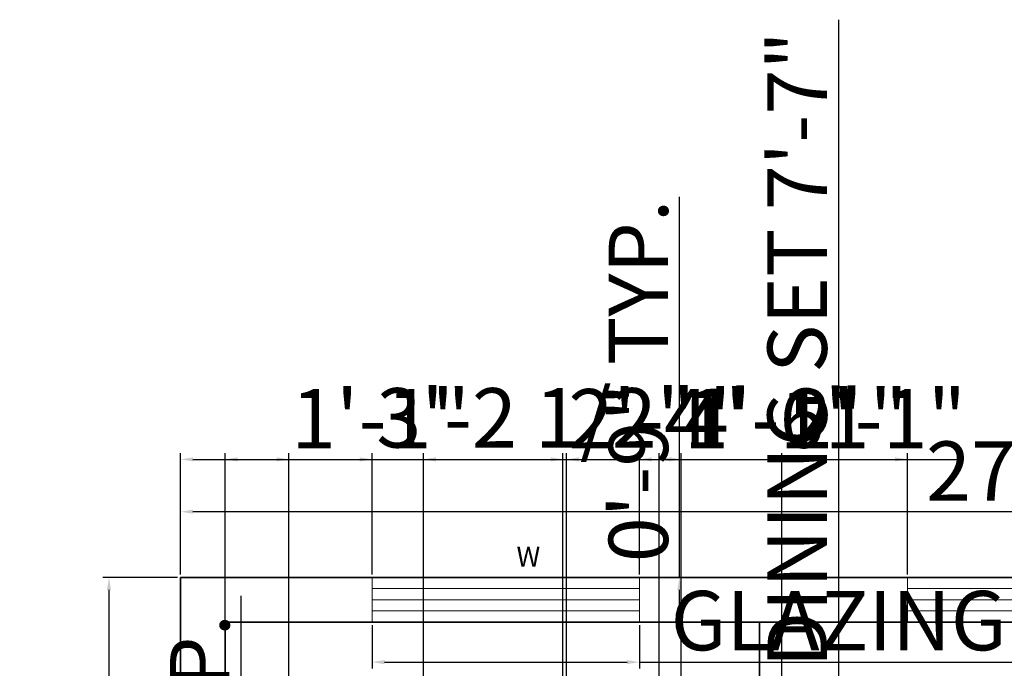
# Model space of a CAD drawing. Units: inches. Extents: x 2691 to 3133, y 1294 to 1993.
# Tile 6 of 7: x 2736 to 2935, y 1862 to 1993. Entities that reach past the tile are written whole.
import ezdxf

# ---------------------------------------------------------------- set-up
doc = ezdxf.new("R2010")
doc.units = ezdxf.units.IN
for name, color, linetype, lineweight in [('A-ANNO-DIMS', 2, 'Continuous', 18), ('A-ANNO-TEXT', 7, 'Continuous', 18), ('A-GLAZ', 4, 'Continuous', 18), ('A-WALL', 7, 'Continuous', 35)]:
    doc.layers.add(name, color=color, linetype=linetype, lineweight=lineweight)
doc.styles.get("Standard").update_dxf_attribs({"font": 'arial.ttf'})
doc.dimstyles.new('ISO-25', dxfattribs={"dimtxt": 12, "dimasz": 2.5, "dimexe": 1.25, "dimexo": 0.625, "dimtad": 1, "dimdec": 1, "dimlunit": 3, "dimtxsty": 'Standard', "dimcen": 2.5, "dimadec": 0, "dimazin": 0, "dimtfac": 1, "dimtdec": 1, "dimtmove": 0, "dimatfit": 3, "dimfxl": 1, "dimarcsym": 0})

# ---------------------------------------------------------------- blocks, each defined once
blk = doc.blocks.new('Window - Wood Frame 36 in. Wide plan')
for p, q in [((0, 6), (0, 0)), ((36, 6), (36, 0)), ((0, 4.5), (36, 4.5)), ((0, 3), (36, 3)), ((0, 1.5), (36, 1.5))]:
    blk.add_line(p, q)
blk = doc.blocks.new('*D10')
at = {"layer": 'A-ANNO-DIMS', "color": 0, "lineweight": -2, "transparency": 16777216}
for p, q in [((2768.25, 1880.68), (2768.25, 1894.58)), ((3092.25, 1880.68), (3092.25, 1894.58)), ((3089.75, 1893.33), (2770.75, 1893.33))]:
    blk.add_line(p, q, dxfattribs=at)
at = {"layer": 'A-ANNO-DIMS', "color": 0, "transparency": 16777216}
for points in [[(2770.75, 1893.75), (2770.75, 1892.92), (2768.25, 1893.33)], [(3089.75, 1893.75), (3089.75, 1892.92), (3092.25, 1893.33)]]:
    blk.add_solid(points, dxfattribs=at)
at = {"layer": 'Defpoints', "color": 0, "transparency": 16777216}
for p in [(2768.25, 1893.33), (2768.25, 1880.05), (3092.25, 1880.05)]:
    blk.add_point(p, dxfattribs=at)
at = {"layer": 'A-ANNO-DIMS', "color": 0, "transparency": 16777216, "insert": (2930.25, 1899.98), "char_height": 12, "attachment_point": 5}
blk.add_mtext("27'", dxfattribs=at)
blk = doc.blocks.new('*D11')
at = {"layer": 'A-ANNO-DIMS', "color": 0, "lineweight": -2, "transparency": 16777216}
for p, q in [((2767.62, 1880.05), (2752.52, 1880.05)), ((2753.77, 1877.55), (2753.77, 1426.55)), ((2767.62, 1424.05), (2752.52, 1424.05))]:
    blk.add_line(p, q, dxfattribs=at)
at = {"layer": 'A-ANNO-DIMS', "color": 0, "transparency": 16777216}
for points in [[(2753.35, 1877.55), (2754.18, 1877.55), (2753.77, 1880.05)], [(2753.35, 1426.55), (2754.18, 1426.55), (2753.77, 1424.05)]]:
    blk.add_solid(points, dxfattribs=at)
at = {"layer": 'Defpoints', "color": 0, "transparency": 16777216}
for p in [(2768.25, 1880.05), (2753.77, 1424.05), (2768.25, 1424.05)]:
    blk.add_point(p, dxfattribs=at)
at = {"layer": 'A-ANNO-DIMS', "color": 0, "transparency": 16777216, "insert": (2747.01, 1652.05), "char_height": 12, "attachment_point": 5, "rotation": 90}
blk.add_mtext("38'", dxfattribs=at)
blk = doc.blocks.new('*D14')
at = {"layer": 'A-ANNO-DIMS', "color": 0, "lineweight": -2, "transparency": 16777216}
for p, q in [((2806.97, 1870.43), (2806.97, 1861.7)), ((2860.97, 1870.43), (2860.97, 1861.7)), ((2809.47, 1862.95), (2858.47, 1862.95)), ((2860.97, 1862.95), (3015.92, 1862.95))]:
    blk.add_line(p, q, dxfattribs=at)
at = {"layer": 'A-ANNO-DIMS', "color": 0, "transparency": 16777216}
for points in [[(2809.47, 1863.37), (2809.47, 1862.54), (2806.97, 1862.95)], [(2858.47, 1863.37), (2858.47, 1862.54), (2860.97, 1862.95)]]:
    blk.add_solid(points, dxfattribs=at)
at = {"layer": 'Defpoints', "color": 0, "transparency": 16777216}
for p in [(2806.97, 1871.05), (2860.97, 1871.05), (2860.97, 1862.95)]:
    blk.add_point(p, dxfattribs=at)
at = {"layer": 'A-ANNO-DIMS', "color": 0, "transparency": 16777216, "insert": (2939.69, 1869.78), "char_height": 12, "attachment_point": 5}
blk.add_mtext('GLAZING 4\'-6" TYP.', dxfattribs=at)
blk = doc.blocks.new('*D15')
at = {"layer": 'A-ANNO-DIMS', "color": 0, "lineweight": -2, "transparency": 16777216}
for p, q in [((2869.07, 1880.05), (2869.07, 1956.95)), ((2861.6, 1880.05), (2870.32, 1880.05)), ((2869.07, 1873.55), (2869.07, 1877.55)), ((2861.6, 1871.05), (2870.32, 1871.05))]:
    blk.add_line(p, q, dxfattribs=at)
at = {"layer": 'A-ANNO-DIMS', "color": 0, "transparency": 16777216}
for points in [[(2868.66, 1877.55), (2869.49, 1877.55), (2869.07, 1880.05)], [(2868.66, 1873.55), (2869.49, 1873.55), (2869.07, 1871.05)]]:
    blk.add_solid(points, dxfattribs=at)
at = {"layer": 'Defpoints', "color": 0, "transparency": 16777216}
for p in [(2860.97, 1880.05), (2869.07, 1880.05), (2860.97, 1871.05)]:
    blk.add_point(p, dxfattribs=at)
at = {"layer": 'A-ANNO-DIMS', "color": 0, "transparency": 16777216, "insert": (2862.32, 1919.75), "char_height": 12, "attachment_point": 5, "rotation": 90}
blk.add_mtext('0\'-9" TYP.', dxfattribs=at)
blk = doc.blocks.new('*D18')
at = {"layer": 'A-ANNO-DIMS', "color": 0, "lineweight": -2, "transparency": 16777216}
for p, q in [((2780.49, 1693.45), (2780.49, 1876.36)), ((2777.87, 1693.45), (2781.74, 1693.45)), ((2780.49, 1674.35), (2780.49, 1690.95)), ((2777.87, 1671.85), (2781.74, 1671.85))]:
    blk.add_line(p, q, dxfattribs=at)
at = {"layer": 'A-ANNO-DIMS', "color": 0, "transparency": 16777216}
for points in [[(2780.07, 1690.95), (2780.91, 1690.95), (2780.49, 1693.45)], [(2780.07, 1674.35), (2780.91, 1674.35), (2780.49, 1671.85)]]:
    blk.add_solid(points, dxfattribs=at)
at = {"layer": 'Defpoints', "color": 0, "transparency": 16777216}
for p in [(2777.25, 1693.45), (2780.49, 1693.45), (2777.25, 1671.85)]:
    blk.add_point(p, dxfattribs=at)
at = {"layer": 'A-ANNO-DIMS', "color": 0, "transparency": 16777216, "insert": (2773.66, 1786.16), "char_height": 12, "attachment_point": 5, "rotation": 90}
blk.add_mtext('GLAZING 1\'-9 1/2" TYP.', dxfattribs=at)
blk = doc.blocks.new('*D30')
at = {"layer": 'A-ANNO-DIMS', "color": 0, "lineweight": -2, "transparency": 16777216}
for p, q in [((2901.25, 1857.07), (2901.25, 1992.71)), ((2914.28, 1857.07), (2900, 1857.07)), ((2901.25, 1768.57), (2901.25, 1854.57)), ((2914.28, 1766.07), (2900, 1766.07))]:
    blk.add_line(p, q, dxfattribs=at)
at = {"layer": 'A-ANNO-DIMS', "color": 0, "transparency": 16777216}
for points in [[(2900.84, 1854.57), (2901.67, 1854.57), (2901.25, 1857.07)], [(2900.84, 1768.57), (2901.67, 1768.57), (2901.25, 1766.07)]]:
    blk.add_solid(points, dxfattribs=at)
at = {"layer": 'Defpoints', "color": 0, "transparency": 16777216}
for p in [(2901.25, 1857.07), (2914.9, 1857.07), (2914.9, 1766.07)]:
    blk.add_point(p, dxfattribs=at)
at = {"layer": 'A-ANNO-DIMS', "color": 0, "transparency": 16777216, "insert": (2894.42, 1926.14), "char_height": 12, "attachment_point": 5, "rotation": 90}
blk.add_mtext('DINING SET 7\'-7"', dxfattribs=at)
blk = doc.blocks.new('*D38')
at = {"layer": 'A-ANNO-DIMS', "color": 0, "lineweight": -2, "transparency": 16777216}
for p, q in [((2768.25, 1880.68), (2768.25, 1905.15)), ((2806.97, 1880.68), (2806.97, 1905.15)), ((2770.75, 1903.9), (2804.47, 1903.9)), ((2806.97, 1903.9), (2870.58, 1903.9))]:
    blk.add_line(p, q, dxfattribs=at)
at = {"layer": 'A-ANNO-DIMS', "color": 0, "transparency": 16777216}
for points in [[(2770.75, 1904.32), (2770.75, 1903.49), (2768.25, 1903.9)], [(2804.47, 1904.32), (2804.47, 1903.49), (2806.97, 1903.9)]]:
    blk.add_solid(points, dxfattribs=at)
at = {"layer": 'Defpoints', "color": 0, "transparency": 16777216}
for p in [(2806.97, 1903.9), (2768.25, 1880.05), (2806.97, 1880.05)]:
    blk.add_point(p, dxfattribs=at)
at = {"layer": 'A-ANNO-DIMS', "color": 0, "transparency": 16777216, "insert": (2840.02, 1910.74), "char_height": 12, "attachment_point": 5}
blk.add_mtext('3\'-2 1/2"', dxfattribs=at)
blk = doc.blocks.new('*D39')
at = {"layer": 'A-ANNO-DIMS', "color": 0, "lineweight": -2, "transparency": 16777216}
for p, q in [((2860.97, 1880.68), (2860.97, 1905.15)), ((2915.15, 1880.68), (2915.15, 1905.15)), ((2863.47, 1903.9), (2912.65, 1903.9))]:
    blk.add_line(p, q, dxfattribs=at)
at = {"layer": 'A-ANNO-DIMS', "color": 0, "transparency": 16777216}
for points in [[(2863.47, 1904.32), (2863.47, 1903.49), (2860.97, 1903.9)], [(2912.65, 1904.32), (2912.65, 1903.49), (2915.15, 1903.9)]]:
    blk.add_solid(points, dxfattribs=at)
at = {"layer": 'Defpoints', "color": 0, "transparency": 16777216}
for p in [(2915.15, 1903.9), (2860.97, 1880.05), (2915.15, 1880.05)]:
    blk.add_point(p, dxfattribs=at)
at = {"layer": 'A-ANNO-DIMS', "color": 0, "transparency": 16777216, "insert": (2888.06, 1910.66), "char_height": 12, "attachment_point": 5}
blk.add_mtext('4\'-6"', dxfattribs=at)
blk = doc.blocks.new('*D54')
at = {"layer": 'A-ANNO-DIMS', "color": 0, "lineweight": -2, "transparency": 16777216}
for p, q in [((2846.25, 1645.18), (2846.25, 1905.15)), ((2869.44, 1645.18), (2869.44, 1905.15)), ((2848.75, 1903.9), (2866.94, 1903.9)), ((2869.44, 1903.9), (2913.28, 1903.9))]:
    blk.add_line(p, q, dxfattribs=at)
at = {"layer": 'A-ANNO-DIMS', "color": 0, "transparency": 16777216}
for points in [[(2848.75, 1904.32), (2848.75, 1903.49), (2846.25, 1903.9)], [(2866.94, 1904.32), (2866.94, 1903.49), (2869.44, 1903.9)]]:
    blk.add_solid(points, dxfattribs=at)
at = {"layer": 'Defpoints', "color": 0, "transparency": 16777216}
for p in [(2869.44, 1903.9), (2846.25, 1644.55), (2869.44, 1644.55)]:
    blk.add_point(p, dxfattribs=at)
at = {"layer": 'A-ANNO-DIMS', "color": 0, "transparency": 16777216, "insert": (2892.61, 1910.55), "char_height": 12, "attachment_point": 5}
blk.add_mtext('1\'-11"', dxfattribs=at)
blk = doc.blocks.new('*D57')
at = {"layer": 'A-ANNO-DIMS', "color": 0, "lineweight": -2, "transparency": 16777216}
for p, q in [((2777.25, 1709.68), (2777.25, 1905.15)), ((2790.15, 1709.61), (2790.15, 1905.15)), ((2779.75, 1903.9), (2787.65, 1903.9)), ((2790.15, 1903.9), (2824.67, 1903.9))]:
    blk.add_line(p, q, dxfattribs=at)
at = {"layer": 'A-ANNO-DIMS', "color": 0, "transparency": 16777216}
for points in [[(2779.75, 1904.32), (2779.75, 1903.49), (2777.25, 1903.9)], [(2787.65, 1904.32), (2787.65, 1903.49), (2790.15, 1903.9)]]:
    blk.add_solid(points, dxfattribs=at)
at = {"layer": 'Defpoints', "color": 0, "transparency": 16777216}
for p in [(2790.15, 1903.9), (2777.25, 1709.05), (2790.15, 1708.98)]:
    blk.add_point(p, dxfattribs=at)
at = {"layer": 'A-ANNO-DIMS', "color": 0, "transparency": 16777216, "insert": (2808.66, 1910.55), "char_height": 12, "attachment_point": 5}
blk.add_mtext('1\'-1"', dxfattribs=at)
blk = doc.blocks.new('*D60')
at = {"layer": 'A-ANNO-DIMS', "color": 0, "lineweight": -2, "transparency": 16777216}
for p, q in [((2817.34, 1781.68), (2817.34, 1905.15)), ((2845.53, 1786.1), (2845.53, 1905.15)), ((2819.84, 1903.9), (2843.03, 1903.9)), ((2845.53, 1903.9), (2881.38, 1903.9))]:
    blk.add_line(p, q, dxfattribs=at)
at = {"layer": 'A-ANNO-DIMS', "color": 0, "transparency": 16777216}
for points in [[(2819.84, 1904.32), (2819.84, 1903.49), (2817.34, 1903.9)], [(2843.03, 1904.32), (2843.03, 1903.49), (2845.53, 1903.9)]]:
    blk.add_solid(points, dxfattribs=at)
at = {"layer": 'Defpoints', "color": 0, "transparency": 16777216}
for p in [(2845.53, 1903.9), (2845.53, 1785.48), (2817.34, 1781.05)]:
    blk.add_point(p, dxfattribs=at)
at = {"layer": 'A-ANNO-DIMS', "color": 0, "transparency": 16777216, "insert": (2864.71, 1910.55), "char_height": 12, "attachment_point": 5}
blk.add_mtext('2\'-4"', dxfattribs=at)
blk = doc.blocks.new('*D61')
at = {"layer": 'A-ANNO-DIMS', "color": 0, "lineweight": -2, "transparency": 16777216}
for p, q in [((2864.96, 1433.88), (2864.96, 1905.15)), ((2889.75, 1433.68), (2889.75, 1905.15)), ((2867.46, 1903.9), (2887.25, 1903.9)), ((2889.75, 1903.9), (2925.6, 1903.9))]:
    blk.add_line(p, q, dxfattribs=at)
at = {"layer": 'A-ANNO-DIMS', "color": 0, "transparency": 16777216}
for points in [[(2867.46, 1904.32), (2867.46, 1903.49), (2864.96, 1903.9)], [(2887.25, 1904.32), (2887.25, 1903.49), (2889.75, 1903.9)]]:
    blk.add_solid(points, dxfattribs=at)
at = {"layer": 'Defpoints', "color": 0, "transparency": 16777216}
for p in [(2889.75, 1903.9), (2864.96, 1433.26), (2889.75, 1433.05)]:
    blk.add_point(p, dxfattribs=at)
at = {"layer": 'A-ANNO-DIMS', "color": 0, "transparency": 16777216, "insert": (2908.93, 1910.55), "char_height": 12, "attachment_point": 5}
blk.add_mtext('2\'-1"', dxfattribs=at)

msp = doc.modelspace()

# ---------------------------------------------------------------- linework, layer by layer
at = {"layer": 'A-WALL'}
for p, q in [((3092.25, 1880.05), (2768.25, 1880.05)), ((2768.25, 1880.05), (2768.25, 1424.05)), ((2777.25, 1871.05), (2777.25, 1761.55)), ((2880.75, 1871.05), (2777.25, 1871.05)), ((3083.25, 1871.05), (2880.75, 1871.05)), ((2885.25, 1796.11), (2885.25, 1871.05))]:
    msp.add_line(p, q, dxfattribs=at)

# ---------------------------------------------------------------- block references
at = {"layer": 'A-GLAZ', "xscale": 1.5, "yscale": 1.5}
for p in [(2806.97, 1871.05), (2915.15, 1871.05)]:
    msp.add_blockref('Window - Wood Frame 36 in. Wide plan', p, dxfattribs=at)

# ---------------------------------------------------------------- texts
at = {"layer": 'A-ANNO-TEXT', "insert": (2836.14, 1886.26), "char_height": 4, "attachment_point": 1}
msp.add_mtext_dynamic_manual_height_columns('W', width=0.1038, gutter_width=12.5, heights=[0], dxfattribs=at)

# ---------------------------------------------------------------- dimensions: what is measured, and where the dimension line sits
at = {"layer": 'A-ANNO-DIMS'}
for base, p1, p2, text, picture, middle in [((2901.25, 1857.07), (2914.9, 1766.07), (2914.9, 1857.07), 'DINING SET <>', '*D30', (2894.42, 1926.14)), ((2869.07, 1880.05), (2860.97, 1871.05), (2860.97, 1880.05), '<> TYP.', '*D15', (2862.32, 1919.75)), ((2780.49, 1693.45), (2777.25, 1671.85), (2777.25, 1693.45), 'GLAZING <> TYP.', '*D18', (2773.66, 1786.16))]:
    dim = msp.add_linear_dim(base=base, p1=p1, p2=p2, angle=90, text=text, dimstyle='ISO-25', override={"dimdec": 1, "dimlfac": 1, "dimrnd": 0, "dimzin": 1, "dimdsep": 46, "dimlunit": 4, "dimfrac": 2}, dxfattribs=at)
    dim.commit()
    dim.dimension.update_dxf_attribs({"geometry": picture, "text_midpoint": middle})
for base, p1, p2, override, picture, middle in [((2806.97, 1903.9), (2768.25, 1880.05), (2806.97, 1880.05), {"dimdec": 1, "dimlfac": 1, "dimrnd": 0, "dimzin": 1, "dimdsep": 46, "dimlunit": 4, "dimfrac": 2}, '*D38', (2840.02, 1910.74)), ((2790.15, 1903.9), (2777.25, 1709.05), (2790.15, 1708.98), {"dimdec": 1, "dimlfac": 1, "dimrnd": 0, "dimzin": 1, "dimdsep": 46, "dimlunit": 4, "dimfrac": 2}, '*D57', (2808.66, 1910.55)), ((2845.53, 1903.9), (2817.34, 1781.05), (2845.53, 1785.48), {"dimdec": 1, "dimlfac": 1, "dimrnd": 0, "dimzin": 1, "dimdsep": 46, "dimlunit": 4, "dimfrac": 2}, '*D60', (2864.71, 1910.55)), ((2869.44, 1903.9), (2846.25, 1644.55), (2869.44, 1644.55), {"dimdec": 1, "dimlfac": 1, "dimrnd": 0, "dimzin": 1, "dimdsep": 46, "dimlunit": 4, "dimfrac": 2}, '*D54', (2892.61, 1910.55)), ((2915.15, 1903.9), (2860.97, 1880.05), (2915.15, 1880.05), {"dimdec": 1, "dimlfac": 1, "dimrnd": 0, "dimzin": 1, "dimdsep": 46, "dimlunit": 4, "dimfrac": 2}, '*D39', (2888.06, 1910.66)), ((2889.75, 1903.9), (2864.96, 1433.26), (2889.75, 1433.05), {"dimdec": 1, "dimlfac": 1, "dimrnd": 0, "dimzin": 1, "dimdsep": 46, "dimlunit": 4, "dimfrac": 2}, '*D61', (2908.93, 1910.55)), ((2768.25, 1893.33), (3092.25, 1880.05), (2768.25, 1880.05), {"dimclrd": 0, "dimclre": 0, "dimclrt": 0}, '*D10', (2930.25, 1899.98))]:
    dim = msp.add_linear_dim(base=base, p1=p1, p2=p2, dimstyle='ISO-25', override=override, dxfattribs=at)
    dim.commit()
    dim.dimension.update_dxf_attribs({"geometry": picture, "text_midpoint": middle})
dim = msp.add_linear_dim(base=(2860.97, 1862.95), p1=(2806.97, 1871.05), p2=(2860.97, 1871.05), text='GLAZING <> TYP.', dimstyle='ISO-25', override={"dimdec": 1, "dimlfac": 1, "dimrnd": 0, "dimzin": 1, "dimdsep": 46, "dimlunit": 4, "dimfrac": 2}, dxfattribs=at)
dim.commit()
dim.dimension.update_dxf_attribs({"geometry": '*D14', "text_midpoint": (2939.69, 1869.78)})
dim = msp.add_linear_dim(base=(2753.77, 1424.05), p1=(2768.25, 1880.05), p2=(2768.25, 1424.05), angle=90, dimstyle='ISO-25', override={"dimclrd": 0, "dimclre": 0, "dimclrt": 0}, dxfattribs=at)
dim.commit()
dim.dimension.update_dxf_attribs({"geometry": '*D11', "text_midpoint": (2747.01, 1652.05)})

doc.saveas('drawing.dxf')
